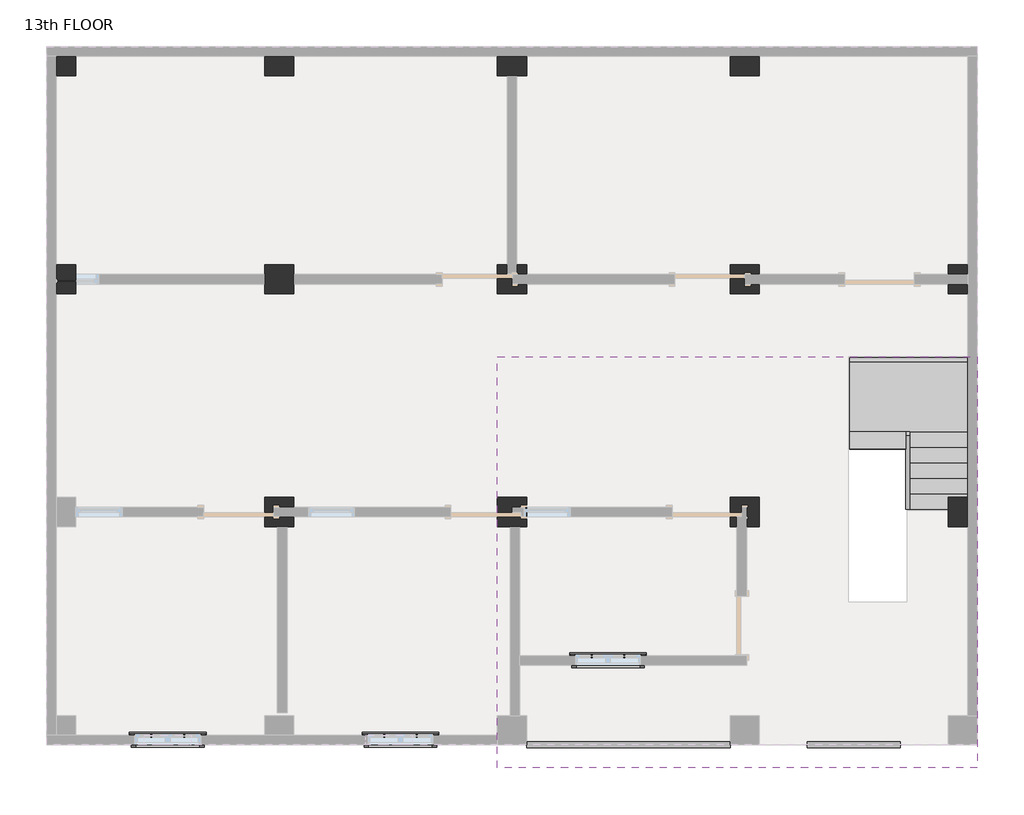
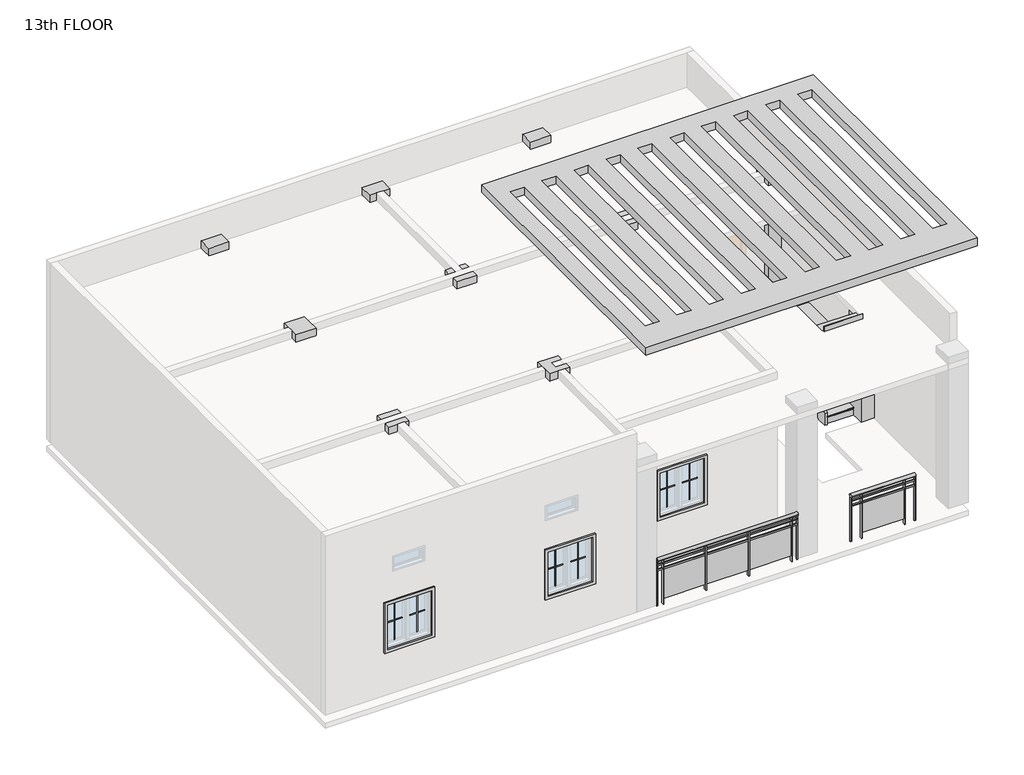
# One storey, part 2 of 2: 13 columns, 12 proxies, 4 members, 2 railings, 1 damper, 1 stair flight.
"""IFC4 building model written with IfcOpenShell, lengths in millimetres."""

from ifc_helpers import new_model, si_unit, point, frame, origin, place, context, project, spatial, polyline, ellipse_curve, trimmed, outline, extrude, faceted_brep, transform, mapped, element, save
from ifc_brep_helpers import plane_surface, extruded_surface, advanced_brep
from components import muntin_pattern_2x2_muntin_pattern_2x2_b3fe6957, muntin_pattern_2x2_muntin_pattern_2x2_3e0ecaf2, trim_window_exterior_flat_with_sill_41619996, trim_window_interior_flat_picture_frame_51c85655, duct_accessories_14_duct_accessories_14_a27dce4f, stair_flight_148faca6

model = new_model("IFC4")

# Units and contexts
model_context = context("Model", 3, world=origin())
ifc_project = project(units=[si_unit("LENGTHUNIT", "METRE", prefix="MILLI")], contexts=[model_context])

# Site, building, storey
site = spatial("IfcSite", under=ifc_project)
building = spatial("IfcBuilding", under=site)
storey = spatial("IfcBuildingStorey", under=building, Name="13th FLOOR", Elevation=39471.6)

# Proxies
placement = place(None, origin())
muntin_pattern_2x2_muntin_pattern_2x2_shape = muntin_pattern_2x2_muntin_pattern_2x2_b3fe6957(model_context)
element("IfcBuildingElementProxy", 1, Name="Muntin Pattern_2x2 : Muntin Pattern_2x2", ObjectType="Muntin Pattern_2x2 : Muntin Pattern_2x2", at=placement, inside=storey, context=model_context, shape_type="MappedRepresentation", body=[
    mapped(muntin_pattern_2x2_muntin_pattern_2x2_shape, transform((-14441.409625, -253.8184478, 40455.85), x_axis=(1.0, 0.0, 0.0), y_axis=(0.0, 1.0, 0.0), z_axis=(0.0, 0.0, 1.0))),
])
element("IfcBuildingElementProxy", 2, Name="Muntin Pattern_2x2 : Muntin Pattern_2x2", ObjectType="Muntin Pattern_2x2 : Muntin Pattern_2x2", at=placement, inside=storey, context=model_context, shape_type="MappedRepresentation", body=[
    mapped(muntin_pattern_2x2_muntin_pattern_2x2_shape, transform((-11393.409625, -253.8184478, 40455.85), x_axis=(1.0, 0.0, 0.0), y_axis=(0.0, 1.0, 0.0), z_axis=(0.0, 0.0, 1.0))),
])
element("IfcBuildingElementProxy", 3, Name="Muntin Pattern_2x2 : Muntin Pattern_2x2", ObjectType="Muntin Pattern_2x2 : Muntin Pattern_2x2", at=placement, inside=storey, context=model_context, shape_type="MappedRepresentation", body=[
    mapped(muntin_pattern_2x2_muntin_pattern_2x2_shape, transform((-8675.609625, 787.5815522, 40455.85), x_axis=(1.0, 0.0, 0.0), y_axis=(0.0, 1.0, 0.0), z_axis=(0.0, 0.0, 1.0))),
])
muntin_pattern_2x2_muntin_pattern_2x2_2_shape = muntin_pattern_2x2_muntin_pattern_2x2_3e0ecaf2(model_context)
element("IfcBuildingElementProxy", 4, Name="Muntin Pattern_2x2 : Muntin Pattern_2x2", ObjectType="Muntin Pattern_2x2 : Muntin Pattern_2x2", at=placement, inside=storey, context=model_context, shape_type="MappedRepresentation", body=[
    mapped(muntin_pattern_2x2_muntin_pattern_2x2_2_shape, transform((-14012.784625, -253.8184478, 40455.85), x_axis=(-1.0, 0.0, 0.0), y_axis=(0.0, -1.0, 0.0), z_axis=(0.0, 0.0, 1.0))),
])
element("IfcBuildingElementProxy", 5, Name="Muntin Pattern_2x2 : Muntin Pattern_2x2", ObjectType="Muntin Pattern_2x2 : Muntin Pattern_2x2", at=placement, inside=storey, context=model_context, shape_type="MappedRepresentation", body=[
    mapped(muntin_pattern_2x2_muntin_pattern_2x2_2_shape, transform((-10964.784625, -253.8184478, 40455.85), x_axis=(-1.0, 0.0, 0.0), y_axis=(0.0, -1.0, 0.0), z_axis=(0.0, 0.0, 1.0))),
])
element("IfcBuildingElementProxy", 6, Name="Muntin Pattern_2x2 : Muntin Pattern_2x2", ObjectType="Muntin Pattern_2x2 : Muntin Pattern_2x2", at=placement, inside=storey, context=model_context, shape_type="MappedRepresentation", body=[
    mapped(muntin_pattern_2x2_muntin_pattern_2x2_2_shape, transform((-8246.984625, 787.5815522, 40455.85), x_axis=(-1.0, 0.0, 0.0), y_axis=(0.0, -1.0, 0.0), z_axis=(0.0, 0.0, 1.0))),
])
trim_window_exterior_flat_with_sill_shape = trim_window_exterior_flat_with_sill_41619996(model_context)
element("IfcBuildingElementProxy", 7, Name="Trim-Window-Exterior-Flat : with Sill", ObjectType="Trim-Window-Exterior-Flat : with Sill", at=placement, inside=storey, context=model_context, shape_type="MappedRepresentation", body=[
    mapped(trim_window_exterior_flat_with_sill_shape, transform((-14227.097125, -244.2934478, 41300.4), x_axis=(-1.0, 0.0, 0.0), y_axis=(0.0, 0.0, 1.0), z_axis=(0.0, 1.0, 0.0))),
])
element("IfcBuildingElementProxy", 8, Name="Trim-Window-Exterior-Flat : with Sill", ObjectType="Trim-Window-Exterior-Flat : with Sill", at=placement, inside=storey, context=model_context, shape_type="MappedRepresentation", body=[
    mapped(trim_window_exterior_flat_with_sill_shape, transform((-11179.097125, -244.2934478, 41300.4), x_axis=(-1.0, 0.0, 0.0), y_axis=(0.0, 0.0, 1.0), z_axis=(0.0, 1.0, 0.0))),
])
element("IfcBuildingElementProxy", 9, Name="Trim-Window-Exterior-Flat : with Sill", ObjectType="Trim-Window-Exterior-Flat : with Sill", at=placement, inside=storey, context=model_context, shape_type="MappedRepresentation", body=[
    mapped(trim_window_exterior_flat_with_sill_shape, transform((-8461.297125, 797.1065522, 41300.4), x_axis=(-1.0, 0.0, 0.0), y_axis=(0.0, 0.0, 1.0), z_axis=(0.0, 1.0, 0.0))),
])
trim_window_interior_flat_picture_frame_shape = trim_window_interior_flat_picture_frame_51c85655(model_context)
element("IfcBuildingElementProxy", 10, Name="Trim-Window-Interior-Flat : Picture Frame", ObjectType="Trim-Window-Interior-Flat : Picture Frame", at=placement, inside=storey, context=model_context, shape_type="MappedRepresentation", body=[
    mapped(trim_window_interior_flat_picture_frame_shape, transform((-14227.097125, -371.2934478, 41300.4), x_axis=(1.0, 0.0, 0.0), y_axis=(0.0, 0.0, 1.0), z_axis=(0.0, -1.0, 0.0))),
])
element("IfcBuildingElementProxy", 11, Name="Trim-Window-Interior-Flat : Picture Frame", ObjectType="Trim-Window-Interior-Flat : Picture Frame", at=placement, inside=storey, context=model_context, shape_type="MappedRepresentation", body=[
    mapped(trim_window_interior_flat_picture_frame_shape, transform((-11179.097125, -371.2934478, 41300.4), x_axis=(1.0, 0.0, 0.0), y_axis=(0.0, 0.0, 1.0), z_axis=(0.0, -1.0, 0.0))),
])
element("IfcBuildingElementProxy", 12, Name="Trim-Window-Interior-Flat : Picture Frame", ObjectType="Trim-Window-Interior-Flat : Picture Frame", at=placement, inside=storey, context=model_context, shape_type="MappedRepresentation", body=[
    mapped(trim_window_interior_flat_picture_frame_shape, transform((-8461.297125, 670.1065522, 41300.4), x_axis=(1.0, 0.0, 0.0), y_axis=(0.0, 0.0, 1.0), z_axis=(0.0, -1.0, 0.0))),
])

# Columns
element("IfcColumn", 13, ObjectType="column family : column family", at=placement, inside=storey, context=model_context, shape_type="SweptSolid", body=[
    extrude(outline(polyline([(-15433.597125, 8645.7065522), (-15433.597125, 8391.7065522), (-15687.597125, 8391.7065522), (-15687.597125, 8645.7065522), (-15433.597125, 8645.7065522)])), frame((0.0, 0.0, 39476.6), z_axis=(0.0, 0.0, 1.0), x_axis=(1.0, 0.0, 0.0)), (0.0, 0.0, 1.0), 3038.0),
])
element("IfcColumn", 14, ObjectType="column family : column family", at=placement, inside=storey, context=model_context, shape_type="SweptSolid", body=[
    extrude(outline(polyline([(-12576.097125, 5915.2065522), (-12576.097125, 5534.2065522), (-12957.097125, 5534.2065522), (-12957.097125, 5915.2065522), (-12576.097125, 5915.2065522)])), frame((0.0, 0.0, 39476.6), z_axis=(0.0, 0.0, 1.0), x_axis=(1.0, 0.0, 0.0)), (0.0, 0.0, 1.0), 3038.0),
])
element("IfcColumn", 15, ObjectType="column family : column family", at=placement, inside=storey, context=model_context, shape_type="Brep", body=[
    faceted_brep([(-9655.097125, 5915.2065522, 39476.6), (-9528.097125, 5915.2065522, 39476.6), (-9528.097125, 5788.2065522, 39476.6), (-9655.097125, 5788.2065522, 39476.6), (-9528.097125, 5915.2065522, 42514.6), (-9655.097125, 5915.2065522, 42514.6), (-9655.097125, 5788.2065522, 42514.6), (-9528.097125, 5788.2065522, 42514.6)], [[[0, 1, 2, 3]], [[4, 5, 6, 7]], [[0, 3, 6, 5]], [[4, 1, 0, 5]], [[3, 2, 7, 6]], [[1, 4, 7, 2]]]),
    faceted_brep([(-9528.097125, 5534.2065522, 42514.6), (-9528.097125, 5534.2065522, 39476.6), (-9528.097125, 5661.2065522, 39476.6), (-9528.097125, 5661.2065522, 42514.6), (-9909.097125, 5534.2065522, 39476.6), (-9909.097125, 5534.2065522, 42514.6), (-9909.097125, 5915.2065522, 39476.6), (-9909.097125, 5661.2065522, 42514.6), (-9909.097125, 5661.2065522, 41605.2), (-9909.097125, 5788.2065522, 41605.2), (-9909.097125, 5788.2065522, 42514.6), (-9909.097125, 5915.2065522, 42514.6), (-9782.097125, 5915.2065522, 42514.6), (-9782.097125, 5915.2065522, 39476.6), (-9782.097125, 5788.2065522, 39476.6), (-9782.097125, 5788.2065522, 42514.6), (-9782.097125, 5788.2065522, 41605.2), (-9718.597125, 5788.2065522, 39476.6), (-9718.597125, 5788.2065522, 41605.2), (-9718.597125, 5661.2065522, 39476.6), (-9718.597125, 5661.2065522, 41605.2)], [[[0, 1, 2, 3]], [[4, 1, 0, 5]], [[6, 4, 5, 7, 8, 9, 10, 11]], [[6, 11, 12, 13]], [[14, 13, 12, 15, 16]], [[17, 14, 16, 18]], [[19, 20, 8, 7, 3, 2]], [[1, 4, 6, 13, 14, 17, 19, 2]], [[5, 0, 3, 7]], [[12, 11, 10, 15]], [[9, 16, 15, 10]], [[18, 20, 19, 17]], [[20, 18, 16, 9, 8]]]),
])
element("IfcColumn", 16, ObjectType="column family : column family", at=placement, inside=storey, context=model_context, shape_type="Brep", body=[
    faceted_brep([(-6480.097125, 5534.2065522, 39476.6), (-6861.097125, 5534.2065522, 39476.6), (-6861.097125, 5915.2065522, 39476.6), (-6480.097125, 5915.2065522, 39476.6), (-6480.097125, 5788.2065522, 39476.6), (-6670.597125, 5788.2065522, 39476.6), (-6670.597125, 5661.2065522, 39476.6), (-6480.097125, 5661.2065522, 39476.6), (-6480.097125, 5534.2065522, 42514.6), (-6480.097125, 5661.2065522, 42514.6), (-6861.097125, 5534.2065522, 42514.6), (-6861.097125, 5661.2065522, 42514.6), (-6861.097125, 5661.2065522, 41605.2), (-6861.097125, 5788.2065522, 41605.2), (-6861.097125, 5788.2065522, 42514.6), (-6861.097125, 5915.2065522, 42514.6), (-6480.097125, 5915.2065522, 42514.6), (-6670.597125, 5661.2065522, 41605.2), (-6670.597125, 5788.2065522, 41605.2), (-6480.097125, 5788.2065522, 42514.6)], [[[0, 1, 2, 3, 4, 5, 6, 7]], [[8, 0, 7, 9]], [[1, 0, 8, 10]], [[2, 1, 10, 11, 12, 13, 14, 15]], [[3, 2, 15, 16]], [[10, 8, 9, 11]], [[6, 17, 12, 11, 9, 7]], [[13, 18, 5, 4, 19, 14]], [[3, 16, 19, 4]], [[16, 15, 14, 19]], [[18, 17, 6, 5]], [[17, 18, 13, 12]]]),
])
element("IfcColumn", 17, ObjectType="column family : column family", at=placement, inside=storey, context=model_context, shape_type="Brep", body=[
    faceted_brep([(-6480.097125, 2867.2065522, 39476.6), (-6480.097125, 2486.2065522, 39476.6), (-6645.197125, 2486.2065522, 39476.6), (-6645.197125, 2740.2065522, 39476.6), (-6708.697125, 2740.2065522, 39476.6), (-6708.697125, 2613.2065522, 39476.6), (-6772.197125, 2613.2065522, 39476.6), (-6772.197125, 2486.2065522, 39476.6), (-6861.097125, 2486.2065522, 39476.6), (-6861.097125, 2867.2065522, 39476.6), (-6480.097125, 2867.2065522, 42514.6), (-6480.097125, 2486.2065522, 42514.6), (-6861.097125, 2486.2065522, 42514.6), (-6772.197125, 2486.2065522, 42514.6), (-6861.097125, 2613.2065522, 42514.6), (-6861.097125, 2613.2065522, 41605.2), (-6861.097125, 2740.2065522, 41605.2), (-6861.097125, 2740.2065522, 42514.6), (-6861.097125, 2867.2065522, 42514.6), (-6772.197125, 2740.2065522, 42514.6), (-6645.197125, 2740.2065522, 42514.6), (-6645.197125, 2486.2065522, 42514.6), (-6772.197125, 2613.2065522, 42514.6), (-6772.197125, 2613.2065522, 41605.2), (-6772.197125, 2740.2065522, 41605.2), (-6708.697125, 2613.2065522, 41605.2), (-6708.697125, 2740.2065522, 41605.2)], [[[0, 1, 2, 3, 4, 5, 6, 7, 8, 9]], [[1, 0, 10, 11]], [[12, 8, 7, 13]], [[9, 8, 12, 14, 15, 16, 17, 18]], [[0, 9, 18, 10]], [[11, 10, 18, 17, 19, 20, 21]], [[15, 14, 22, 23]], [[17, 16, 24, 19]], [[20, 3, 2, 21]], [[6, 23, 22, 13, 7]], [[14, 12, 13, 22]], [[1, 11, 21, 2]], [[15, 23, 24, 16]], [[25, 23, 6, 5]], [[23, 25, 26, 24]], [[26, 25, 5, 4]], [[24, 26, 4, 3, 20, 19]]]),
])
element("IfcColumn", 18, ObjectType="column family : column family", at=placement, inside=storey, context=model_context, shape_type="Brep", body=[
    faceted_brep([(-9528.097125, 2486.2065522, 39476.6), (-9909.097125, 2486.2065522, 39476.6), (-9909.097125, 2867.2065522, 39476.6), (-9528.097125, 2867.2065522, 39476.6), (-9528.097125, 2740.2065522, 39476.6), (-9566.197125, 2740.2065522, 39476.6), (-9718.597125, 2740.2065522, 39476.6), (-9718.597125, 2613.2065522, 39476.6), (-9566.197125, 2613.2065522, 39476.6), (-9528.097125, 2613.2065522, 39476.6), (-9528.097125, 2486.2065522, 42514.6), (-9528.097125, 2613.2065522, 39776.4), (-9528.097125, 2740.2065522, 39776.4), (-9528.097125, 2867.2065522, 42514.6), (-9528.097125, 2740.2065522, 42514.6), (-9528.097125, 2740.2065522, 41605.2), (-9528.097125, 2613.2065522, 41605.2), (-9528.097125, 2613.2065522, 42514.6), (-9909.097125, 2486.2065522, 42514.6), (-9909.097125, 2867.2065522, 42514.6), (-9566.197125, 2613.2065522, 42514.6), (-9718.597125, 2613.2065522, 42514.6), (-9718.597125, 2740.2065522, 42514.6), (-9566.197125, 2740.2065522, 42514.6), (-9566.197125, 2613.2065522, 41605.2), (-9566.197125, 2613.2065522, 39776.4), (-9566.197125, 2740.2065522, 39776.4), (-9566.197125, 2740.2065522, 41605.2)], [[[0, 1, 2, 3, 4, 5, 6, 7, 8, 9]], [[10, 0, 9, 11, 12, 4, 3, 13, 14, 15, 16, 17]], [[1, 0, 10, 18]], [[2, 1, 18, 19]], [[3, 2, 19, 13]], [[18, 10, 17, 20, 21, 22, 23, 14, 13, 19]], [[11, 9, 8, 7, 21, 20, 17, 16, 24, 25]], [[4, 12, 26, 27, 15, 14, 23, 22, 6, 5]], [[21, 7, 6, 22]], [[25, 24, 27, 26]], [[25, 26, 12, 11]], [[27, 24, 16, 15]]]),
])
element("IfcColumn", 19, ObjectType="column family : column family", at=placement, inside=storey, context=model_context, shape_type="Brep", body=[
    faceted_brep([(-12576.097125, 2486.2065522, 39476.6), (-12957.097125, 2486.2065522, 39476.6), (-12957.097125, 2867.2065522, 39476.6), (-12576.097125, 2867.2065522, 39476.6), (-12576.097125, 2740.2065522, 39476.6), (-12842.797125, 2740.2065522, 39476.6), (-12842.797125, 2613.2065522, 39476.6), (-12576.097125, 2613.2065522, 39476.6), (-12576.097125, 2486.2065522, 42514.6), (-12576.097125, 2613.2065522, 42514.6), (-12957.097125, 2486.2065522, 42514.6), (-12957.097125, 2613.2065522, 42514.6), (-12957.097125, 2613.2065522, 41605.2), (-12957.097125, 2740.2065522, 41605.2), (-12957.097125, 2740.2065522, 42514.6), (-12957.097125, 2867.2065522, 42514.6), (-12576.097125, 2867.2065522, 42514.6), (-12842.797125, 2613.2065522, 41605.2), (-12842.797125, 2740.2065522, 41605.2), (-12576.097125, 2740.2065522, 42514.6)], [[[0, 1, 2, 3, 4, 5, 6, 7]], [[8, 0, 7, 9]], [[1, 0, 8, 10]], [[2, 1, 10, 11, 12, 13, 14, 15]], [[3, 2, 15, 16]], [[10, 8, 9, 11]], [[6, 17, 12, 11, 9, 7]], [[13, 18, 5, 4, 19, 14]], [[3, 16, 19, 4]], [[16, 15, 14, 19]], [[17, 18, 13, 12]], [[18, 17, 6, 5]]]),
])
element("IfcColumn", 20, ObjectType="column family : column family", at=placement, inside=storey, context=model_context, shape_type="SweptSolid", body=[
    extrude(outline(polyline([(-12576.097125, 8391.7065522), (-12957.097125, 8391.7065522), (-12957.097125, 8645.7065522), (-12576.097125, 8645.7065522), (-12576.097125, 8391.7065522)])), frame((0.0, 0.0, 39476.6), z_axis=(0.0, 0.0, 1.0), x_axis=(1.0, 0.0, 0.0)), (0.0, 0.0, 1.0), 3038.0),
])
element("IfcColumn", 21, ObjectType="column family : column family", at=placement, inside=storey, context=model_context, shape_type="SweptSolid", body=[
    extrude(outline(polyline([(-9528.097125, 8391.7065522), (-9909.097125, 8391.7065522), (-9909.097125, 8645.7065522), (-9528.097125, 8645.7065522), (-9528.097125, 8391.7065522)])), frame((0.0, 0.0, 39476.6), z_axis=(0.0, 0.0, 1.0), x_axis=(1.0, 0.0, 0.0)), (0.0, 0.0, 1.0), 3038.0),
])
element("IfcColumn", 22, ObjectType="column family : column family", at=placement, inside=storey, context=model_context, shape_type="SweptSolid", body=[
    extrude(outline(polyline([(-6480.097125, 8391.7065522), (-6861.097125, 8391.7065522), (-6861.097125, 8645.7065522), (-6480.097125, 8645.7065522), (-6480.097125, 8391.7065522)])), frame((0.0, 0.0, 39476.6), z_axis=(0.0, 0.0, 1.0), x_axis=(1.0, 0.0, 0.0)), (0.0, 0.0, 1.0), 3038.0),
])
element("IfcColumn", 23, ObjectType="column family : column family", at=placement, inside=storey, context=model_context, shape_type="SweptSolid", body=[
    extrude(outline(polyline([(-4003.597125, 5915.2065522), (-3749.597125, 5915.2065522), (-3749.597125, 5788.2065522), (-4003.597125, 5788.2065522), (-4003.597125, 5915.2065522)])), frame((0.0, 0.0, 39476.6), z_axis=(0.0, 0.0, 1.0), x_axis=(1.0, 0.0, 0.0)), (0.0, 0.0, 1.0), 3038.0),
    extrude(outline(polyline([(-3749.597125, 5534.2065522), (-4003.597125, 5534.2065522), (-4003.597125, 5661.2065522), (-3749.597125, 5661.2065522), (-3749.597125, 5534.2065522)])), frame((0.0, 0.0, 39476.6), z_axis=(0.0, 0.0, 1.0), x_axis=(1.0, 0.0, 0.0)), (0.0, 0.0, 1.0), 3038.0),
])
element("IfcColumn", 24, ObjectType="column family : column family", at=placement, inside=storey, context=model_context, shape_type="SweptSolid", body=[
    extrude(outline(polyline([(-4003.597125, 2486.2065522), (-4003.597125, 2867.2065522), (-3749.597125, 2867.2065522), (-3749.597125, 2486.2065522), (-4003.597125, 2486.2065522)])), frame((0.0, 0.0, 39476.6), z_axis=(0.0, 0.0, 1.0), x_axis=(1.0, 0.0, 0.0)), (0.0, 0.0, 1.0), 3038.0),
])
element("IfcColumn", 25, ObjectType="column family : column family", at=placement, inside=storey, context=model_context, shape_type="SweptSolid", body=[
    extrude(outline(polyline([(-15433.597125, 5915.2065522), (-15433.597125, 5534.2065522), (-15687.597125, 5534.2065522), (-15687.597125, 5915.2065522), (-15433.597125, 5915.2065522)])), frame((0.0, 0.0, 39476.6), z_axis=(0.0, 0.0, 1.0), x_axis=(1.0, 0.0, 0.0)), (0.0, 0.0, 1.0), 3038.0),
])

# Damper
duct_accessories_14_duct_accessories_14_shape = duct_accessories_14_duct_accessories_14_a27dce4f(model_context)
element("IfcDamper", 26, ObjectType="Duct Accessories 14 : Duct Accessories 14", at=placement, inside=storey, context=model_context, shape_type="MappedRepresentation", body=[
    mapped(duct_accessories_14_duct_accessories_14_shape, transform((0.0, 0.0, 0.0), x_axis=(1.0, 0.0, 0.0), y_axis=(0.0, 1.0, 0.0), z_axis=(0.0, 0.0, 1.0))),
])

# Members
element("IfcMember", 27, ObjectType="Stringer - 2\" Width", at=placement, inside=storey, context=model_context, shape_type="SweptSolid", body=[
    extrude(outline(polyline([(2714.6319226, 39471.6), (2714.6319226, 39708.4438745), (3679.8319226, 40512.7772078), (3679.8319226, 40116.0165243), (2906.5320935, 39471.6), (2714.6319226, 39471.6)])), frame((-4563.0136682, 0.0, 0.0), z_axis=(1.0, 0.0, 0.0), x_axis=(0.0, 1.0, 0.0)), (0.0, 0.0, 1.0), 50.8),
])
element("IfcMember", 28, ObjectType="Stringer - 2\" Width", at=placement, inside=storey, context=model_context, shape_type="SweptSolid", body=[
    extrude(outline(polyline([(-4512.2136682, 3730.6319226), (-4512.2136682, 3679.8319226), (-4563.0136682, 3679.8319226), (-4563.0136682, 3730.6319226), (-4512.2136682, 3730.6319226)])), frame((0.0, 0.0, 40259.0), z_axis=(0.0, 0.0, 1.0), x_axis=(1.0, 0.0, 0.0)), (0.0, 0.0, 1.0), 304.8),
])
element("IfcMember", 29, ObjectType="Stringer - 2\" Width", at=placement, inside=storey, context=model_context, shape_type="SweptSolid", body=[
    extrude(outline(polyline([(2714.6319226, 39471.6), (2714.6319226, 39708.4438745), (3741.0592732, 40563.8), (4217.1720935, 40563.8), (2906.5320935, 39471.6), (2714.6319226, 39471.6)])), frame((-3749.597125, 0.0, 0.0), z_axis=(1.0, 0.0, 0.0), x_axis=(0.0, 1.0, 0.0)), (0.0, 0.0, 1.0), 50.8),
])
element("IfcMember", 30, ObjectType="Stringer - 2\" Width", at=placement, inside=storey, context=model_context, shape_type="SweptSolid", body=[
    extrude(outline(polyline([(-3698.797125, 4695.8319226), (-3698.797125, 4645.0319226), (-5295.0246464, 4645.0319226), (-5295.0246464, 4695.8319226), (-3698.797125, 4695.8319226)])), frame((0.0, 0.0, 40259.0), z_axis=(0.0, 0.0, 1.0), x_axis=(1.0, 0.0, 0.0)), (0.0, 0.0, 1.0), 304.8),
])

# Railings
element("IfcRailing", 31, ObjectType="Glass Panel - Bottom Fill", at=placement, inside=storey, context=model_context, shape_type="SolidModel", body=[
    advanced_brep(
    [(-9528.097125, -333.1934478, 40386.0), (-9528.097125, -409.3934478, 40386.0), (-6861.097125, -333.1934478, 40386.0), (-6861.097125, -409.3934478, 40386.0)],
    [
        (0, 1, ellipse_curve(frame((-9528.097125, -371.2934478, 40386.0), z_axis=(-1.0, 0.0, 0.0), x_axis=(0.0, -1.0, 0.0)), 38.1, 28.575)),
        (1, 0, ellipse_curve(frame((-9528.097125, -371.2934478, 40386.0), z_axis=(-1.0, 0.0, 0.0), x_axis=(0.0, -1.0, 0.0)), 38.1, 28.575)),
        (2, 3, ellipse_curve(frame((-6861.097125, -371.2934478, 40386.0), z_axis=(1.0, 0.0, 0.0), x_axis=(0.0, -1.0, 0.0)), 38.1, 28.575)),
        (3, 2, ellipse_curve(frame((-6861.097125, -371.2934478, 40386.0), z_axis=(1.0, 0.0, 0.0), x_axis=(0.0, -1.0, 0.0)), 38.1, 28.575)),
        (0, 2),
        (3, 1),
    ],
    [
        plane_surface(frame((-9528.097125, -371.2934478, 40386.0), z_axis=(-1.0, 0.0, 0.0), x_axis=(0.0, 1.0, 0.0))),
        plane_surface(frame((-6861.097125, -371.2934478, 40386.0), z_axis=(1.0, 0.0, 0.0), x_axis=(0.0, 1.0, 0.0))),
        extruded_surface(trimmed(ellipse_curve(frame((-6861.097125, -371.2934478, 40386.0), z_axis=(-1.0, 0.0, 0.0), x_axis=(0.0, -1.0, 0.0)), 38.1, 28.575), [point((-6861.097125, -333.1934478, 40386.0))], [point((-6861.097125, -409.3934478, 40386.0))], True, "CARTESIAN"), (-2667.0, 0.0, 0.0), 2667.0),
        extruded_surface(trimmed(ellipse_curve(frame((-6861.097125, -371.2934478, 40386.0), z_axis=(-1.0, 0.0, 0.0), x_axis=(0.0, -1.0, 0.0)), 38.1, 28.575), [point((-6861.097125, -409.3934478, 40386.0))], [point((-6861.097125, -333.1934478, 40386.0))], True, "CARTESIAN"), (-2667.0, 0.0, 0.0), 2667.0),
    ],
    [
        (0, [[1, 2]]),
        (1, [[3, 4]]),
        (2, [[-1, 5, -4, 6]]),
        (3, [[-2, -6, -3, -5]]),
    ],
),
    extrude(outline(polyline([(-9528.097125, -383.9934478), (-9528.097125, -358.5934478), (-6861.097125, -358.5934478), (-6861.097125, -383.9934478), (-9528.097125, -383.9934478)])), frame((0.0, 0.0, 40271.7), z_axis=(0.0, 0.0, 1.0), x_axis=(1.0, 0.0, 0.0)), (0.0, 0.0, 1.0), 25.4),
    extrude(outline(polyline([(-9528.097125, -383.9934478), (-9528.097125, -358.5934478), (-6861.097125, -358.5934478), (-6861.097125, -383.9934478), (-9528.097125, -383.9934478)])), frame((0.0, 0.0, 40170.1), z_axis=(0.0, 0.0, 1.0), x_axis=(1.0, 0.0, 0.0)), (0.0, 0.0, 1.0), 25.4),
    extrude(outline(polyline([(-6981.747125, -396.6934478), (-6981.747125, -345.8934478), (-6969.047125, -345.8934478), (-6969.047125, -396.6934478), (-6981.747125, -396.6934478)])), frame((0.0, 0.0, 39471.6), z_axis=(0.0, 0.0, 1.0), x_axis=(1.0, 0.0, 0.0)), (0.0, 0.0, 1.0), 885.6788223),
    extrude(outline(polyline([(-7788.197125, -364.7582908), (-6975.397125, -364.7582908), (-6975.397125, -371.1082908), (-7788.197125, -371.1082908), (-7788.197125, -364.7582908)])), frame((0.0, 0.0, 39573.2), z_axis=(0.0, 0.0, 1.0), x_axis=(1.0, 0.0, 0.0)), (0.0, 0.0, 1.0), 596.9),
    extrude(outline(polyline([(-7794.547125, -396.6934478), (-7794.547125, -345.8934478), (-7781.847125, -345.8934478), (-7781.847125, -396.6934478), (-7794.547125, -396.6934478)])), frame((0.0, 0.0, 39471.6), z_axis=(0.0, 0.0, 1.0), x_axis=(1.0, 0.0, 0.0)), (0.0, 0.0, 1.0), 885.6788223),
    extrude(outline(polyline([(-8600.997125, -364.7582908), (-7788.197125, -364.7582908), (-7788.197125, -371.1082908), (-8600.997125, -371.1082908), (-8600.997125, -364.7582908)])), frame((0.0, 0.0, 39573.2), z_axis=(0.0, 0.0, 1.0), x_axis=(1.0, 0.0, 0.0)), (0.0, 0.0, 1.0), 596.9),
    extrude(outline(polyline([(-8607.347125, -396.6934478), (-8607.347125, -345.8934478), (-8594.647125, -345.8934478), (-8594.647125, -396.6934478), (-8607.347125, -396.6934478)])), frame((0.0, 0.0, 39471.6), z_axis=(0.0, 0.0, 1.0), x_axis=(1.0, 0.0, 0.0)), (0.0, 0.0, 1.0), 885.6788223),
    extrude(outline(polyline([(-9413.797125, -364.7582908), (-8600.997125, -364.7582908), (-8600.997125, -371.1082908), (-9413.797125, -371.1082908), (-9413.797125, -364.7582908)])), frame((0.0, 0.0, 39573.2), z_axis=(0.0, 0.0, 1.0), x_axis=(1.0, 0.0, 0.0)), (0.0, 0.0, 1.0), 596.9),
    extrude(outline(polyline([(-9420.147125, -396.6934478), (-9420.147125, -345.8934478), (-9407.447125, -345.8934478), (-9407.447125, -396.6934478), (-9420.147125, -396.6934478)])), frame((0.0, 0.0, 39471.6), z_axis=(0.0, 0.0, 1.0), x_axis=(1.0, 0.0, 0.0)), (0.0, 0.0, 1.0), 885.6788223),
    extrude(outline(polyline([(-6873.797125, -380.8184478), (-6873.797125, -361.7684478), (-6854.747125, -361.7684478), (-6854.747125, -380.8184478), (-6873.797125, -380.8184478)])), frame((0.0, 0.0, 39471.6), z_axis=(0.0, 0.0, 1.0), x_axis=(1.0, 0.0, 0.0)), (0.0, 0.0, 1.0), 885.6788223),
    extrude(outline(polyline([(-9534.447125, -380.8184478), (-9534.447125, -361.7684478), (-9515.397125, -361.7684478), (-9515.397125, -380.8184478), (-9534.447125, -380.8184478)])), frame((0.0, 0.0, 39471.6), z_axis=(0.0, 0.0, 1.0), x_axis=(1.0, 0.0, 0.0)), (0.0, 0.0, 1.0), 885.6788223),
])
element("IfcRailing", 32, ObjectType="Glass Panel - Bottom Fill", at=placement, inside=storey, context=model_context, shape_type="SolidModel", body=[
    advanced_brep(
    [(-5851.447125, -333.1934478, 40386.0), (-5851.447125, -409.3934478, 40386.0), (-4632.247125, -333.1934478, 40386.0), (-4632.247125, -409.3934478, 40386.0)],
    [
        (0, 1, ellipse_curve(frame((-5851.447125, -371.2934478, 40386.0), z_axis=(-1.0, 0.0, 0.0), x_axis=(0.0, -1.0, 0.0)), 38.1, 28.575)),
        (1, 0, ellipse_curve(frame((-5851.447125, -371.2934478, 40386.0), z_axis=(-1.0, 0.0, 0.0), x_axis=(0.0, -1.0, 0.0)), 38.1, 28.575)),
        (2, 3, ellipse_curve(frame((-4632.247125, -371.2934478, 40386.0), z_axis=(1.0, 0.0, 0.0), x_axis=(0.0, -1.0, 0.0)), 38.1, 28.575)),
        (3, 2, ellipse_curve(frame((-4632.247125, -371.2934478, 40386.0), z_axis=(1.0, 0.0, 0.0), x_axis=(0.0, -1.0, 0.0)), 38.1, 28.575)),
        (0, 2),
        (3, 1),
    ],
    [
        plane_surface(frame((-5851.447125, -371.2934478, 40386.0), z_axis=(-1.0, 0.0, 0.0), x_axis=(0.0, 1.0, 0.0))),
        plane_surface(frame((-4632.247125, -371.2934478, 40386.0), z_axis=(1.0, 0.0, 0.0), x_axis=(0.0, 1.0, 0.0))),
        extruded_surface(trimmed(ellipse_curve(frame((-4632.247125, -371.2934478, 40386.0), z_axis=(-1.0, 0.0, 0.0), x_axis=(0.0, -1.0, 0.0)), 38.1, 28.575), [point((-4632.247125, -333.1934478, 40386.0))], [point((-4632.247125, -409.3934478, 40386.0))], True, "CARTESIAN"), (-1219.1999999999998, 0.0, 0.0), 1219.1999999999998),
        extruded_surface(trimmed(ellipse_curve(frame((-4632.247125, -371.2934478, 40386.0), z_axis=(-1.0, 0.0, 0.0), x_axis=(0.0, -1.0, 0.0)), 38.1, 28.575), [point((-4632.247125, -409.3934478, 40386.0))], [point((-4632.247125, -333.1934478, 40386.0))], True, "CARTESIAN"), (-1219.1999999999998, 0.0, 0.0), 1219.1999999999998),
    ],
    [
        (0, [[1, 2]]),
        (1, [[3, 4]]),
        (2, [[-1, 5, -4, 6]]),
        (3, [[-2, -6, -3, -5]]),
    ],
),
    extrude(outline(polyline([(-5851.447125, -383.9934478), (-5851.447125, -358.5934478), (-4632.247125, -358.5934478), (-4632.247125, -383.9934478), (-5851.447125, -383.9934478)])), frame((0.0, 0.0, 40271.7), z_axis=(0.0, 0.0, 1.0), x_axis=(1.0, 0.0, 0.0)), (0.0, 0.0, 1.0), 25.4),
    extrude(outline(polyline([(-5851.447125, -383.9934478), (-5851.447125, -358.5934478), (-4632.247125, -358.5934478), (-4632.247125, -383.9934478), (-5851.447125, -383.9934478)])), frame((0.0, 0.0, 40170.1), z_axis=(0.0, 0.0, 1.0), x_axis=(1.0, 0.0, 0.0)), (0.0, 0.0, 1.0), 25.4),
    extrude(outline(polyline([(-4841.797125, -396.6934478), (-4841.797125, -345.8934478), (-4829.097125, -345.8934478), (-4829.097125, -396.6934478), (-4841.797125, -396.6934478)])), frame((0.0, 0.0, 39471.6), z_axis=(0.0, 0.0, 1.0), x_axis=(1.0, 0.0, 0.0)), (0.0, 0.0, 1.0), 885.6788223),
    extrude(outline(polyline([(-5648.247125, -364.7582908), (-4835.447125, -364.7582908), (-4835.447125, -371.1082908), (-5648.247125, -371.1082908), (-5648.247125, -364.7582908)])), frame((0.0, 0.0, 39573.2), z_axis=(0.0, 0.0, 1.0), x_axis=(1.0, 0.0, 0.0)), (0.0, 0.0, 1.0), 596.9),
    extrude(outline(polyline([(-5654.597125, -396.6934478), (-5654.597125, -345.8934478), (-5641.897125, -345.8934478), (-5641.897125, -396.6934478), (-5654.597125, -396.6934478)])), frame((0.0, 0.0, 39471.6), z_axis=(0.0, 0.0, 1.0), x_axis=(1.0, 0.0, 0.0)), (0.0, 0.0, 1.0), 885.6788223),
    extrude(outline(polyline([(-4644.947125, -380.8184478), (-4644.947125, -361.7684478), (-4625.897125, -361.7684478), (-4625.897125, -380.8184478), (-4644.947125, -380.8184478)])), frame((0.0, 0.0, 39471.6), z_axis=(0.0, 0.0, 1.0), x_axis=(1.0, 0.0, 0.0)), (0.0, 0.0, 1.0), 885.6788223),
    extrude(outline(polyline([(-5857.797125, -380.8184478), (-5857.797125, -361.7684478), (-5838.747125, -361.7684478), (-5838.747125, -380.8184478), (-5857.797125, -380.8184478)])), frame((0.0, 0.0, 39471.6), z_axis=(0.0, 0.0, 1.0), x_axis=(1.0, 0.0, 0.0)), (0.0, 0.0, 1.0), 885.6788223),
])

# Stair flight
stair_flight_shape = stair_flight_148faca6(model_context)
element("IfcStairFlight", 33, ObjectType="2\" Tread 1\" Nosing 1/4\" Riser", at=placement, inside=storey, context=model_context, shape_type="MappedRepresentation", body=[
    mapped(stair_flight_shape, transform((0.0, 0.0, 0.0), x_axis=(1.0, 0.0, 0.0), y_axis=(0.0, 1.0, 0.0), z_axis=(0.0, 0.0, 1.0))),
])

save(model, "model.ifc")

# Revit data of these elements
# Type "Muntin Pattern_2x2 : Muntin Pattern_2x2"
#   Width [instance default] = 4' - 0"
#   Thickness = 0' - 0 1/2"
#   Height [instance default] = 4' - 0"
#   Distance = 0' - 0 3/4"
#   Interior Material [instance default] = none
#   Exterior Material [instance default] = none
#   Default Elevation = 0
# Type "Trim-Window-Exterior-Flat : with Sill"
#   Trim Width = 0' - 2 1/4"
#   Trim Thickness_Picture Frame = 0' - 1 1/4"
#   Trim Thickness_with Sill = 0' - 0 3/4"
#   Sill Thickness = 0' - 1 1/4"
#   Opening Width [instance default] = 2' - 0"
#   Opening Height [instance default] = 3' - 0"
#   Default Elevation = 4' - 0"
#   Sill = yes
#   Picture Frame = no
#   Trim Material [instance default] = none
# Type "Trim-Window-Interior-Flat : Picture Frame"
#   Trim Thickness_Picture Frame = 0' - 1 1/4"
#   Trim Width = 0' - 2 1/4"
#   Trim Thickness_with Sill = 0' - 0 3/4"
#   Sill Thickness = 0' - 1 1/4"
#   Opening Width [instance default] = 2' - 0"
#   Opening Height [instance default] = 3' - 0"
#   Default Elevation = 4' - 0"
#   Sill = no
#   Picture Frame = yes
#   Trim Material [instance default] = none
# Type "column family : column family"
#   w2 [instance default] = 0' - 9.88189"
#   w1 [instance default] = 0' - 9.01575"
#   Depth = 1' - 11.62205"
#   Width = 1' - 11.62205"
# Type "Glass Panel - Bottom Fill"
#   Assembly Code = "C2010400"
#   built-in parameter 1008612 = 0.0416667 (stored number, unit not read)
#   built-in parameter 1008611 = 0.0416667 (stored number, unit not read)
#   built-in parameter 1008609 = 0.333333 (stored number, unit not read)
#   built-in parameter 1008604 = 0.166667 (stored number, unit not read)
#   built-in parameter 1008603 = 0.166667 (stored number, unit not read)
#   Railing Height = 3' - 0"
#   built-in parameter 1008630 = 2
#   built-in parameter 1008610 = 2
#   built-in parameter 1008618 = Baluster - Square : 3/4"
# Elements 1, 2, 3, 4, 5, 6 (IfcBuildingElementProxy, "Muntin Pattern_2x2 : Muntin Pattern_2x2")
#   Width = 0' - 11 5/8"
#   Height = 2' - 6 1/2"
#   Interior Material = Wood - Stained
#   Exterior Material = Clad - White
#   Phase Created = New Construction
#   Materials on its faces: "Clad - White", "Wood - Stained"
# Elements 7, 8, 9 (IfcBuildingElementProxy, "Trim-Window-Exterior-Flat : with Sill")
#   Opening Width = 2' - 10"
#   Opening Height = 3' - 0"
#   Trim Material = Clad - White
#   Phase Created = New Construction
#   Materials on its faces: "Clad - White"
# Elements 10, 11, 12 (IfcBuildingElementProxy, "Trim-Window-Interior-Flat : Picture Frame")
#   Opening Width = 2' - 10"
#   Opening Height = 3' - 0"
#   Trim Material = Wood - Stained
#   Phase Created = New Construction
#   Materials on its faces: "Wood - Stained"
# Elements 13, 14, 15, 20, 21, 22 (IfcColumn, "column family : column family")
#   w2 = 1' - 3"
#   w1 = 1' - 3"
#   Phase Created = New Construction
#   Materials on its faces: "Default Wall"
# Elements 16, 23, 24 (IfcColumn, "column family : column family")
#   w2 = 1' - 3"
#   w1 = 1' - 3"
#   Phase Created = New Construction
#   Materials on its faces: "grey", "Default Wall"
# Element 17 (IfcColumn, "column family : column family")
#   w2 = 1' - 3"
#   w1 = 1' - 3"
#   Phase Created = New Construction
#   Materials on its faces: "Default Wall", "grey", "inside wall"
# Elements 18, 19 (IfcColumn, "column family : column family")
#   w2 = 1' - 3"
#   w1 = 1' - 3"
#   Phase Created = New Construction
#   Materials on its faces: "Default Wall", "inside wall"
# Element 25 (IfcColumn, "column family : column family")
#   w2 = 1' - 3"
#   w1 = 1' - 3"
#   Phase Created = New Construction
#   Materials on its faces: "inside wall", "Default Wall"
# Element 26 (IfcDamper, "Duct Accessories 14 : Duct Accessories 14")
#   Mark = "14"
#   Phase Created = New Construction
#   Materials on its faces: "Clad - White"
# Elements 27, 28, 29, 30 (IfcMember, "Stringer - 2\" Width")
#   Phase Created = New Construction
# Elements 31, 32 (IfcRailing, "Glass Panel - Bottom Fill")
#   Phase Created = New Construction
#   Materials on its faces: "Glass"
# Element 33 (IfcStairFlight, "2\" Tread 1\" Nosing 1/4\" Riser")
#   Phase Created = New Construction
# Materials
#   "Clad - White": class "Wood", colour RGB 242 242 238, transparency 0, Cost = 0
#   "Wood - Stained": class "Wood", colour RGB 224 178 126, transparency 0, Cost = 0
#   "Default Wall": colour RGB 128 128 128, transparency 0, Cost = 0
#   "grey": class "Generic", colour RGB 80 80 80, transparency 0, Cost = 0
#   "inside wall": class "Generic", colour RGB 199 224 95, transparency 0, Cost = 0
#   "Glass": class "Glass", colour RGB 0 128 192, transparency 0.75, Description = "Soda Lime Glass", Cost = 0
